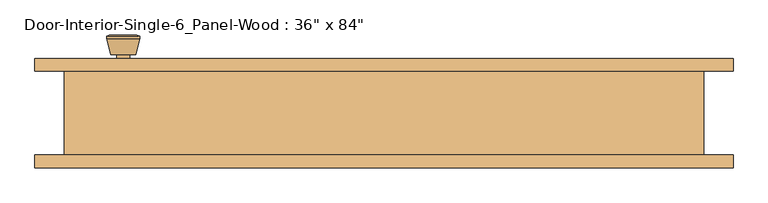
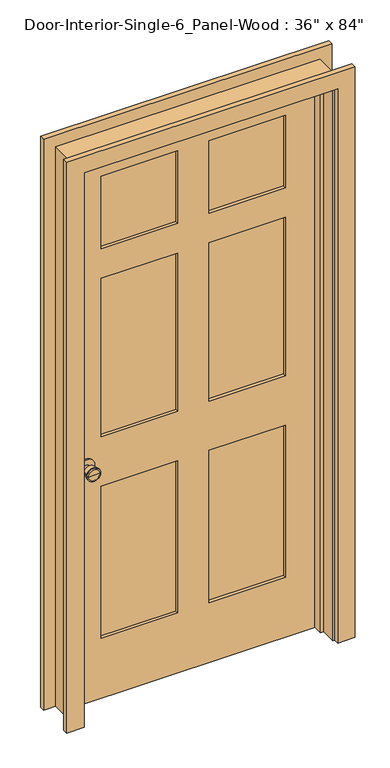
"""IFC4 building model written with IfcOpenShell, lengths in millimetres: door geometry."""

from ifc_helpers import new_model, si_unit, point, frame, frame_2d, origin, place, context, project, spatial, polyline, circle_curve, trimmed, segment, composite_curve, outline, extrude, faceted_brep, source, transform, mapped, element, save
from ifc_brep_helpers import plane_surface, cylinder_surface, revolved_surface, advanced_brep


def door_03e3dfb5(model_context):
    return source(origin(), model_context, "Body", "SolidModel", [
        advanced_brep(
        [(-393.7, 19.4, 914.4), (-383.7, 19.4, 914.4), (-403.7, 19.4, 914.4), (-373.2241324, -29.6, 914.4), (-393.7, -29.6, 914.4), (-414.1758676, -29.6, 914.4), (-368.7, -27.7721319, 914.4), (-418.7, -27.7721319, 914.4), (-368.7, -24.3084537, 914.4), (-418.7, -24.3084537, 914.4), (-375.063764, 0.4, 914.4), (-412.336236, 0.4, 914.4), (-383.7, 0.4, 914.4), (-403.7, 0.4, 914.4)],
        [
            (0, 1),
            (1, 2, circle_curve(frame((-393.7, 19.4, 914.4), z_axis=(0.0, 1.0, 0.0), x_axis=(-1.0, 0.0, 0.0)), 10.0)),
            (2, 0),
            (2, 1, circle_curve(frame((-393.7, 19.4, 914.4), z_axis=(0.0, 1.0, 0.0), x_axis=(-1.0, 0.0, 0.0)), 10.0)),
            (3, 4),
            (4, 5),
            (5, 3, circle_curve(frame((-393.7, -29.6, 914.4), z_axis=(0.0, -1.0, 0.0), x_axis=(-1.0, 0.0, 0.0)), 20.4758676)),
            (3, 5, circle_curve(frame((-393.7, -29.6, 914.4), z_axis=(0.0, -1.0, 0.0), x_axis=(-1.0, 0.0, 0.0)), 20.4758676)),
            (6, 3),
            (5, 7),
            (7, 6, circle_curve(frame((-393.7, -27.7721319, 914.4), z_axis=(0.0, -1.0, 0.0), x_axis=(-1.0, 0.0, 0.0)), 25.0)),
            (6, 7, circle_curve(frame((-393.7, -27.7721319, 914.4), z_axis=(0.0, -1.0, 0.0), x_axis=(-1.0, 0.0, 0.0)), 25.0)),
            (8, 6),
            (7, 9),
            (9, 8, circle_curve(frame((-393.7, -24.3084537, 914.4), z_axis=(0.0, -1.0, 0.0), x_axis=(-1.0, 0.0, 0.0)), 25.0)),
            (8, 9, circle_curve(frame((-393.7, -24.3084537, 914.4), z_axis=(0.0, -1.0, 0.0), x_axis=(-1.0, 0.0, 0.0)), 25.0)),
            (10, 8),
            (9, 11),
            (11, 10, circle_curve(frame((-393.7, 0.4, 914.4), z_axis=(0.0, -1.0, 0.0), x_axis=(-1.0, 0.0, 0.0)), 18.636236)),
            (10, 11, circle_curve(frame((-393.7, 0.4, 914.4), z_axis=(0.0, -1.0, 0.0), x_axis=(-1.0, 0.0, 0.0)), 18.636236)),
            (12, 10),
            (11, 13),
            (13, 12, circle_curve(frame((-393.7, 0.4, 914.4), z_axis=(0.0, -1.0, 0.0), x_axis=(-1.0, 0.0, 0.0)), 10.0)),
            (12, 13, circle_curve(frame((-393.7, 0.4, 914.4), z_axis=(0.0, -1.0, 0.0), x_axis=(-1.0, 0.0, 0.0)), 10.0)),
            (1, 12),
            (13, 2),
        ],
        [
            plane_surface(frame((-393.7, 19.4, 914.4), z_axis=(0.0, 1.0, 0.0), x_axis=(-1.0, 0.0, 0.0))),
            plane_surface(frame((-393.7, -29.6, 914.4), z_axis=(0.0, -1.0, 0.0), x_axis=(-1.0, 0.0, 0.0))),
            revolved_surface(polyline([(-414.1758676, -29.6, 914.4), (-418.7, -27.7721319, 914.4)]), (-393.7, 19.4, 914.4), (0.0, 1.0, 0.0)),
            cylinder_surface(frame((-393.7, 19.4, 914.4), z_axis=(0.0, 1.0, 0.0), x_axis=(-1.0, 0.0, 0.0)), 25.0),
            revolved_surface(polyline([(-418.7, -24.3084537, 914.4), (-412.336236, 0.4, 914.4)]), (-393.7, 19.4, 914.4), (0.0, 1.0, 0.0)),
            plane_surface(frame((-393.7, 0.4, 914.4), z_axis=(0.0, 1.0, 0.0), x_axis=(-1.0, 0.0, 0.0))),
            cylinder_surface(frame((-393.7, 19.4, 914.4), z_axis=(0.0, 1.0, 0.0), x_axis=(-1.0, 0.0, 0.0)), 10.0),
        ],
        [
            (0, [[1, 2, 3]]),
            (0, [[-3, 4, -1]]),
            (1, [[5, 6, 7]]),
            (1, [[-6, -5, 8]]),
            (2, [[9, -7, 10, 11]]),
            (2, [[-10, -8, -9, 12]]),
            (3, [[13, -11, 14, 15]]),
            (3, [[-14, -12, -13, 16]]),
            (4, [[17, -15, 18, 19]]),
            (4, [[-18, -16, -17, 20]]),
            (5, [[21, -19, 22, 23]]),
            (5, [[-22, -20, -21, 24]]),
            (6, [[25, -23, 26, -2]]),
            (6, [[-26, -24, -25, -4]]),
        ],
    ),
        extrude(outline(composite_curve([segment(trimmed(circle_curve(frame_2d((914.4, -393.7)), 30.0), [point((914.4, -423.7))], [point((914.4, -363.7))], False, "CARTESIAN"), True, "CONTINUOUS"), segment(trimmed(circle_curve(frame_2d((914.4, -393.7)), 30.0), [point((914.4, -363.7))], [point((914.4, -423.7))], False, "CARTESIAN"), True, "CONTINUOUS")], self_intersect=False)), frame((0.0, 19.4, 0.0), z_axis=(0.0, 1.0, 0.0), x_axis=(0.0, 0.0, 1.0)), (0.0, 0.0, 1.0), 6.0),
        advanced_brep(
        [(-393.7, 66.325, 914.4), (-403.7, 66.325, 914.4), (-383.7, 66.325, 914.4), (-373.2241324, 115.325, 914.4), (-414.1758676, 115.325, 914.4), (-393.7, 115.325, 914.4), (-368.7, 113.4971319, 914.4), (-418.7, 113.4971319, 914.4), (-368.7, 110.0334537, 914.4), (-418.7, 110.0334537, 914.4), (-375.063764, 85.325, 914.4), (-412.336236, 85.325, 914.4), (-383.7, 85.325, 914.4), (-403.7, 85.325, 914.4)],
        [
            (0, 1),
            (1, 2, circle_curve(frame((-393.7, 66.325, 914.4), z_axis=(0.0, -1.0, 0.0), x_axis=(-1.0, 0.0, 0.0)), 10.0)),
            (2, 0),
            (2, 1, circle_curve(frame((-393.7, 66.325, 914.4), z_axis=(0.0, -1.0, 0.0), x_axis=(-1.0, 0.0, 0.0)), 10.0)),
            (3, 4, circle_curve(frame((-393.7, 115.325, 914.4), z_axis=(0.0, 1.0, 0.0), x_axis=(-1.0, 0.0, 0.0)), 20.4758676)),
            (4, 5),
            (5, 3),
            (4, 3, circle_curve(frame((-393.7, 115.325, 914.4), z_axis=(0.0, 1.0, 0.0), x_axis=(-1.0, 0.0, 0.0)), 20.4758676)),
            (6, 7, circle_curve(frame((-393.7, 113.4971319, 914.4), z_axis=(0.0, 1.0, 0.0), x_axis=(-1.0, 0.0, 0.0)), 25.0)),
            (7, 4),
            (3, 6),
            (7, 6, circle_curve(frame((-393.7, 113.4971319, 914.4), z_axis=(0.0, 1.0, 0.0), x_axis=(-1.0, 0.0, 0.0)), 25.0)),
            (8, 9, circle_curve(frame((-393.7, 110.0334537, 914.4), z_axis=(0.0, 1.0, 0.0), x_axis=(-1.0, 0.0, 0.0)), 25.0)),
            (9, 7),
            (6, 8),
            (9, 8, circle_curve(frame((-393.7, 110.0334537, 914.4), z_axis=(0.0, 1.0, 0.0), x_axis=(-1.0, 0.0, 0.0)), 25.0)),
            (10, 11, circle_curve(frame((-393.7, 85.325, 914.4), z_axis=(0.0, 1.0, 0.0), x_axis=(-1.0, 0.0, 0.0)), 18.636236)),
            (11, 9),
            (8, 10),
            (11, 10, circle_curve(frame((-393.7, 85.325, 914.4), z_axis=(0.0, 1.0, 0.0), x_axis=(-1.0, 0.0, 0.0)), 18.636236)),
            (12, 13, circle_curve(frame((-393.7, 85.325, 914.4), z_axis=(0.0, 1.0, 0.0), x_axis=(-1.0, 0.0, 0.0)), 10.0)),
            (13, 11),
            (10, 12),
            (13, 12, circle_curve(frame((-393.7, 85.325, 914.4), z_axis=(0.0, 1.0, 0.0), x_axis=(-1.0, 0.0, 0.0)), 10.0)),
            (1, 13),
            (12, 2),
        ],
        [
            plane_surface(frame((-393.7, 66.325, 914.4), z_axis=(0.0, -1.0, 0.0), x_axis=(-1.0, 0.0, 0.0))),
            plane_surface(frame((-393.7, 115.325, 914.4), z_axis=(0.0, 1.0, 0.0), x_axis=(-1.0, 0.0, 0.0))),
            revolved_surface(polyline([(-414.1758676, 115.325, 914.4), (-418.7, 113.4971319, 914.4)]), (-393.7, 66.325, 914.4), (0.0, -1.0, 0.0)),
            cylinder_surface(frame((-393.7, 66.325, 914.4), z_axis=(0.0, -1.0, 0.0), x_axis=(-1.0, 0.0, 0.0)), 25.0),
            revolved_surface(polyline([(-418.7, 110.0334537, 914.4), (-412.336236, 85.325, 914.4)]), (-393.7, 66.325, 914.4), (0.0, -1.0, 0.0)),
            plane_surface(frame((-393.7, 85.325, 914.4), z_axis=(0.0, -1.0, 0.0), x_axis=(-1.0, 0.0, 0.0))),
            cylinder_surface(frame((-393.7, 66.325, 914.4), z_axis=(0.0, -1.0, 0.0), x_axis=(-1.0, 0.0, 0.0)), 10.0),
        ],
        [
            (0, [[1, 2, 3]]),
            (0, [[-3, 4, -1]]),
            (1, [[5, 6, 7]]),
            (1, [[8, -7, -6]]),
            (2, [[9, 10, -5, 11]]),
            (2, [[12, -11, -8, -10]]),
            (3, [[13, 14, -9, 15]]),
            (3, [[16, -15, -12, -14]]),
            (4, [[17, 18, -13, 19]]),
            (4, [[20, -19, -16, -18]]),
            (5, [[21, 22, -17, 23]]),
            (5, [[24, -23, -20, -22]]),
            (6, [[-2, 25, -21, 26]]),
            (6, [[-4, -26, -24, -25]]),
        ],
    ),
        extrude(outline(composite_curve([segment(trimmed(circle_curve(frame_2d((914.4, -393.7)), 30.0), [point((914.4, -423.7))], [point((914.4, -363.7))], False, "CARTESIAN"), True, "CONTINUOUS"), segment(trimmed(circle_curve(frame_2d((914.4, -393.7)), 30.0), [point((914.4, -363.7))], [point((914.4, -423.7))], False, "CARTESIAN"), True, "CONTINUOUS")], self_intersect=False)), frame((0.0, 60.325, 0.0), z_axis=(0.0, 1.0, 0.0), x_axis=(0.0, 0.0, 1.0)), (0.0, 0.0, 1.0), 6.0),
        faceted_brep([(482.6, 60.325, 0.0), (482.6, -66.675, 0.0), (457.2, -66.675, 0.0), (457.2, -9.525, 0.0), (444.5, -9.525, 0.0), (444.5, 25.4, 0.0), (457.2, 25.4, 0.0), (457.2, 60.325, 0.0), (482.6, 60.325, 2159.0), (482.6, -66.675, 2159.0), (-482.6, -66.675, 2159.0), (-482.6, -66.675, 0.0), (-457.2, -66.675, 0.0), (-457.2, -66.675, 2133.6), (457.2, -66.675, 2133.6), (457.2, -9.525, 2133.6), (-457.2, -9.525, 2133.6), (-457.2, -9.525, 0.0), (-444.5, -9.525, 0.0), (-444.5, -9.525, 2120.9), (444.5, -9.525, 2120.9), (444.5, 25.4, 2120.9), (-444.5, 25.4, 2120.9), (-444.5, 25.4, 0.0), (-457.2, 25.4, 0.0), (-457.2, 25.4, 2133.6), (457.2, 25.4, 2133.6), (457.2, 60.325, 2133.6), (-457.2, 60.325, 2133.6), (-457.2, 60.325, 0.0), (-482.6, 60.325, 0.0), (-482.6, 60.325, 2159.0)], [[[0, 1, 2, 3, 4, 5, 6, 7]], [[1, 0, 8, 9]], [[2, 1, 9, 10, 11, 12, 13, 14]], [[3, 2, 14, 15]], [[4, 3, 15, 16, 17, 18, 19, 20]], [[5, 4, 20, 21]], [[6, 5, 21, 22, 23, 24, 25, 26]], [[7, 6, 26, 27]], [[0, 7, 27, 28, 29, 30, 31, 8]], [[9, 8, 31, 10]], [[15, 14, 13, 16]], [[21, 20, 19, 22]], [[27, 26, 25, 28]], [[30, 29, 24, 23, 18, 17, 12, 11]], [[10, 31, 30, 11]], [[16, 13, 12, 17]], [[22, 19, 18, 23]], [[28, 25, 24, 29]]]),
        extrude(outline(polyline([(2133.6, -457.2), (0.0, -457.2), (0.0, 457.2), (2133.6, 457.2), (2133.6, -457.2)]), holes=[polyline([(2014.5375, 57.15), (2014.5375, 336.55), (1735.1375, 336.55), (1735.1375, 57.15), (2014.5375, 57.15)]), polyline([(1620.8375, 336.55), (1009.65, 336.55), (1009.65, 57.15), (1620.8375, 57.15), (1620.8375, 336.55)]), polyline([(1009.65, -57.15), (1009.65, -336.55), (1620.8375, -336.55), (1620.8375, -57.15), (1009.65, -57.15)]), polyline([(1735.1375, -336.55), (2014.5375, -336.55), (2014.5375, -57.15), (1735.1375, -57.15), (1735.1375, -336.55)]), polyline([(819.15, 57.15), (819.15, 336.55), (231.775, 336.55), (231.775, 57.15), (819.15, 57.15)]), polyline([(231.775, -57.15), (231.775, -336.55), (819.15, -336.55), (819.15, -57.15), (231.775, -57.15)])]), frame((0.0, 25.4, 0.0), z_axis=(0.0, 1.0, 0.0), x_axis=(0.0, 0.0, 1.0)), (0.0, 0.0, 1.0), 34.925),
        extrude(outline(polyline([(336.55, 37.0416667), (57.15, 37.0416667), (57.15, 48.6833333), (336.55, 48.6833333), (336.55, 37.0416667)])), frame((0.0, 0.0, 1735.1375), z_axis=(0.0, 0.0, 1.0), x_axis=(1.0, 0.0, 0.0)), (0.0, 0.0, 1.0), 279.4),
        extrude(outline(polyline([(336.55, 37.0416667), (57.15, 37.0416667), (57.15, 48.6833333), (336.55, 48.6833333), (336.55, 37.0416667)])), frame((0.0, 0.0, 1009.65), z_axis=(0.0, 0.0, 1.0), x_axis=(1.0, 0.0, 0.0)), (0.0, 0.0, 1.0), 611.1875),
        extrude(outline(polyline([(-57.15, 37.0416667), (-336.55, 37.0416667), (-336.55, 48.6833333), (-57.15, 48.6833333), (-57.15, 37.0416667)])), frame((0.0, 0.0, 1009.65), z_axis=(0.0, 0.0, 1.0), x_axis=(1.0, 0.0, 0.0)), (0.0, 0.0, 1.0), 611.1875),
        extrude(outline(polyline([(-57.15, 37.0416667), (-336.55, 37.0416667), (-336.55, 48.6833333), (-57.15, 48.6833333), (-57.15, 37.0416667)])), frame((0.0, 0.0, 1735.1375), z_axis=(0.0, 0.0, 1.0), x_axis=(1.0, 0.0, 0.0)), (0.0, 0.0, 1.0), 279.4),
        extrude(outline(polyline([(336.55, 37.0416667), (57.15, 37.0416667), (57.15, 48.6833333), (336.55, 48.6833333), (336.55, 37.0416667)])), frame((0.0, 0.0, 231.775), z_axis=(0.0, 0.0, 1.0), x_axis=(1.0, 0.0, 0.0)), (0.0, 0.0, 1.0), 587.375),
        extrude(outline(polyline([(-57.15, 37.0416667), (-336.55, 37.0416667), (-336.55, 48.6833333), (-57.15, 48.6833333), (-57.15, 37.0416667)])), frame((0.0, 0.0, 231.775), z_axis=(0.0, 0.0, 1.0), x_axis=(1.0, 0.0, 0.0)), (0.0, 0.0, 1.0), 587.375),
        extrude(outline(polyline([(0.0, 463.55), (0.0, 527.05), (2203.45, 527.05), (2203.45, -527.05), (0.0, -527.05), (0.0, -463.55), (2139.95, -463.55), (2139.95, 463.55), (0.0, 463.55)])), frame((0.0, 60.325, 0.0), z_axis=(0.0, 1.0, 0.0), x_axis=(0.0, 0.0, 1.0)), (0.0, 0.0, 1.0), 19.05),
        extrude(outline(polyline([(0.0, 463.55), (0.0, 527.05), (2203.45, 527.05), (2203.45, -527.05), (0.0, -527.05), (0.0, -463.55), (2139.95, -463.55), (2139.95, 463.55), (0.0, 463.55)])), frame((0.0, -85.725, 0.0), z_axis=(0.0, 1.0, 0.0), x_axis=(0.0, 0.0, 1.0)), (0.0, 0.0, 1.0), 19.05),
    ])


if __name__ == "__main__":
    model = new_model("IFC4")
    model_context = context("Model", 3, world=origin())
    ifc_project = project(units=[si_unit("LENGTHUNIT", "METRE", prefix="MILLI")], contexts=[model_context])
    site = spatial("IfcSite", under=ifc_project)
    building = spatial("IfcBuilding", under=site)
    placement = place(None, origin())
    door_shape = door_03e3dfb5(model_context)
    element("IfcDoor", 1, ObjectType="Door-Interior-Single-6_Panel-Wood : 36\" x 84\"", at=placement, inside=building, context=model_context, shape_type="MappedRepresentation", body=[
        mapped(door_shape, transform((0.0, 0.0, 0.0), x_axis=(1.0, 0.0, 0.0), y_axis=(0.0, 1.0, 0.0), z_axis=(0.0, 0.0, 1.0))),
    ])
    save(model, "model.ifc")

# Revit data of these elements
# Type "Door-Interior-Single-6_Panel-Wood : 36\" x 84\""
#   Type Mark = "12"
#   Assembly Code = "C1020300"
#   Analytic Construction = "Wooden"
#   Top Rail = 0' - 4 11/16"
#   Top Panel = 0' - 11"
#   Thickness = 0' - 1 3/8"
#   Thermal Resistance (R) = 2.5876 (h·ft²·°F)/BTU
#   Swing Angle [instance default] = 90.00°
#   Stiles = 0' - 4 3/4"
#   Rough Width = 3' - 2"
#   Rough Height = 7' - 1"
#   Mullion = 0' - 4 1/2"
#   Lock Rail = 0' - 7 1/2"
#   Intermediate Rail = 0' - 4 1/2"
#   Height = 7' - 0"
#   Width = 3' - 0"
#   Heat Transfer Coefficient (U) = 0.3865 BTU/(h·ft²·°F)
#   Bottom Rail = 0' - 9 1/8"
#   Trim Material = Cherry
#   Panel Material = Cherry
#   Frame Material = Cherry
#   Door Handle Material = Aluminum
#   Visual Light Transmittance = 0
#   Solar Heat Gain Coefficient = 0
#   Wall Closure = (empty or 0)
#   Function = (empty or 0)
# Element 1 (IfcDoor, "Door-Interior-Single-6_Panel-Wood : 36\" x 84\"")
#   Materials on its faces: "Cherry", "Aluminum"
# Materials
#   "Cherry": class "Wood", colour RGB 226 177 128, transparency 0, Description = "Prunus Serotina", Cost = 0
#   "Aluminum": class "Metal", colour RGB 247 247 247, transparency 0, Description = "Aluminum 6061", Cost = 0
